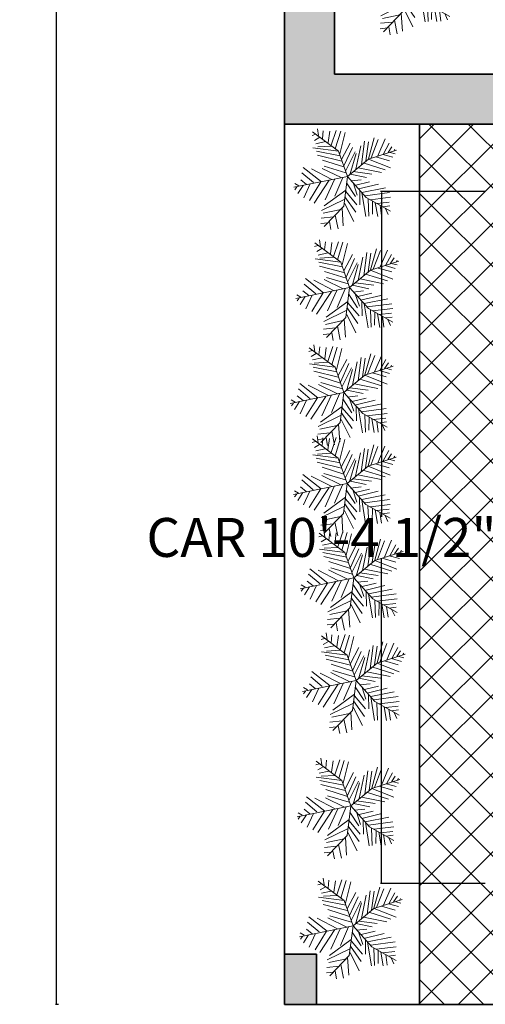
# Model space of a CAD drawing. Units: inches. Extents: x 2167 to 2589, y 1680 to 2489.
# Tile 1 of 38: x 2167 to 2251, y 1688 to 1865. Entities that reach past the tile are written whole.
import ezdxf

# ---------------------------------------------------------------- set-up
doc = ezdxf.new("R2010")
doc.units = ezdxf.units.IN
doc.header["$MEASUREMENT"] = 0
doc.layers.get('0').update_dxf_attribs({"color": 250})
for name, color, linetype, lineweight in [('A-ANNO-DIMS', 2, 'Continuous', 18), ('A-WALL-PATT', 250, 'Continuous', 13), ('C-PROP', 7, 'Continuous', 35), ('L-PLNT', 106, 'Continuous', 13), ('L-PVMT-PATT', 252, 'Continuous', 13), ('walls', 7, 'Continuous', 35)]:
    doc.layers.add(name, color=color, linetype=linetype, lineweight=lineweight)
doc.styles.get("Standard").update_dxf_attribs({"font": 'arial.ttf'})
doc.dimstyles.get("Standard").update_dxf_attribs({"dimtxt": 7, "dimasz": 0.18, "dimexe": 0.18, "dimexo": 0.0625, "dimgap": 0.09, "dimtad": 0, "dimtih": 1, "dimtoh": 1, "dimdec": 1, "dimzin": 0, "dimdsep": 46, "dimlunit": 3, "dimtxsty": 'Standard', "dimcen": 0.09, "dimadec": 0, "dimazin": 0, "dimtfac": 1, "dimtdec": 1, "dimtofl": 0, "dimtmove": 0, "dimatfit": 3, "dimfxl": 1, "dimtolj": 1, "dimtzin": 0, "dimarcsym": 0})

# ---------------------------------------------------------------- blocks, each defined once
blk = doc.blocks.new('*U8')
for p, q in [((-8.737, 47.138), (-17.069, 52.711)), ((-10.186, 53.64), (-13.084, 55.962)), ((0, 0), (-10.5, 57)), ((-9.099, 51.782), (-6.563, 55.962)), ((-7.288, 39.707), (-21.778, 46.673)), ((-7.65, 43.423), (-2.578, 49.46)), ((-5.839, 35.992), (4.667, 48.067)), ((-5.114, 27.632), (10.463, 46.673)), ((-3.665, 19.273), (-27.574, 35.527)), ((-5.114, 28.097), (-24.676, 40.636)), ((-2.941, 16.486), (8.652, 37.85)), ((16.259, 5.805), (23.142, 31.348)), ((22.055, 7.198), (27.489, 32.277)), ((27, 9), (48, 36)), ((27.127, 9.056), (31.112, 35.992)), ((35.096, 32.741), (37.27, 22.524)), ((38.719, 34.134), (41.979, 28.561)), ((44.153, 36.456), (45.239, 32.741)), ((-31.5, 4.5), (-52.5, 25.5)), ((-48.585, 21.131), (-49.309, 29.026)), ((-43.513, 28.561), (-42.427, 15.558)), ((-38.442, 26.239), (-34.819, 7.663)), ((-35.544, 28.097), (-24.314, 3.947)), ((-14.533, 2.09), (-30.834, 25.31)), ((-24.314, 23.917), (-2.941, 13.7)), ((-1.129, 6.734), (9.014, 26.704)), ((3.942, 1.625), (11.187, 24.381)), ((10.101, 3.483), (17.708, 26.239)), ((31.836, 30.883), (32.561, 16.486)), ((40.53, 25.775), (48.862, 24.846)), ((43.791, 29.954), (51.036, 30.883)), ((-47.498, 19.737), (-55.83, 18.344)), ((-40.615, 13.7), (-55.105, 10.913)), ((-20.691, 13.7), (-1.129, 4.876)), ((29.662, 12.307), (48.137, 6.269)), ((33.285, 16.486), (48.862, 10.913)), ((36.183, 19.737), (48.137, 17.88)), ((-33.37, 6.269), (-52.207, 5.34)), ((-28.299, 3.483), (-47.86, -5.805)), ((-21.416, 3.018), (-38.079, -8.128)), ((0, 0), (-31.5, 4.5)), ((-15.982, 2.09), (-30.11, -9.521)), ((0, 0), (-22.5, -19.5)), ((-6.563, 1.161), (-21.416, -8.128)), ((0, 0), (27, 9)), ((0, 0), (18, -22.5)), ((6.478, 1.625), (26.04, -8.592)), ((11.187, 3.483), (30.749, -5.805)), ((18.07, 5.805), (35.096, -3.483)), ((24.229, 7.663), (46.688, 1.625)), ((-6.563, -5.805), (-19.967, -9.985)), ((-9.461, -8.592), (-6.201, -23.453)), ((-4.752, -3.483), (-3.665, -14.629)), ((2.493, -3.019), (-1.491, -20.202)), ((1.769, -2.555), (24.229, -9.521)), ((5.029, -6.27), (2.131, -25.775)), ((7.565, -9.056), (32.198, -14.629)), ((-17.431, -15.094), (-42.789, -18.809)), ((-22.5, -19.5), (-37.5, -45)), ((-15.257, -12.772), (-30.11, -12.772)), ((-20.691, -18.345), (-17.793, -44.352)), ((-17.069, -15.094), (-12.721, -40.172)), ((-13.446, -11.378), (-8.737, -32.741)), ((9.014, -11.378), (3.58, -35.992)), ((14.085, -16.951), (6.478, -40.172)), ((12.274, -15.094), (36.907, -18.809)), ((16.259, -19.738), (36.183, -22.989)), ((-28.299, -29.026), (-42.789, -31.348)), ((-24.314, -21.596), (-42.427, -22.06)), ((-26.849, -26.24), (-40.253, -25.775)), ((-29.023, -30.884), (-27.936, -43.887)), ((-25.038, -23.918), (-22.865, -45.281)), ((18.07, -22.524), (8.289, -45.745)), ((20.244, -30.419), (15.897, -44.816)), ((18, -22.5), (27, -52.5)), ((18.433, -22.524), (40.53, -29.026)), ((19.157, -25.311), (38.719, -33.206)), ((-30.834, -34.135), (-42.427, -35.528)), ((-34.457, -39.708), (-40.978, -42.494)), ((-32.646, -36.921), (-31.921, -44.352)), ((22.78, -37.85), (19.519, -48.532)), ((21.331, -32.741), (39.081, -40.636)), ((22.78, -38.314), (34.372, -44.816)), ((24.591, -45.745), (23.142, -50.854)), ((24.591, -43.423), (30.749, -47.603)), ((26.764, -49.925), (28.213, -50.854))]:
    blk.add_line(p, q)
blk = doc.blocks.new('*D24')
at = {"layer": 'A-ANNO-DIMS', "color": 0, "lineweight": -2, "transparency": 16777216}
for p, q in [((2174.43, 2407.69), (2173.89, 2407.69)), ((2174.07, 2407.51), (2174.07, 2051.36)), ((2174.07, 1687.87), (2174.07, 2044.03)), ((2174.43, 1687.69), (2173.89, 1687.69))]:
    blk.add_line(p, q, dxfattribs=at)
at = {"layer": 'A-ANNO-DIMS', "color": 0, "transparency": 16777216}
for points in [[(2174.04, 2407.51), (2174.1, 2407.51), (2174.07, 2407.69)], [(2174.04, 1687.87), (2174.1, 1687.87), (2174.07, 1687.69)]]:
    blk.add_solid(points, dxfattribs=at)
at = {"layer": 'Defpoints', "color": 0, "transparency": 16777216}
for p in [(2174.49, 2407.69), (2174.07, 1687.69), (2174.49, 1687.69)]:
    blk.add_point(p, dxfattribs=at)
at = {"layer": 'A-ANNO-DIMS', "color": 0, "transparency": 16777216, "insert": (2174.07, 2047.69), "char_height": 7, "attachment_point": 5}
blk.add_mtext("\\A1;60'", dxfattribs=at)
blk = doc.blocks.new('*D45')
at = {"layer": 'A-ANNO-DIMS', "color": 0, "lineweight": -2, "transparency": 16777216}
for p, q in [((2251.16, 1833.95), (2232.36, 1833.95)), ((2232.54, 1833.77), (2232.54, 1775.4)), ((2232.54, 1709.6), (2232.54, 1767.98)), ((2251.16, 1709.42), (2232.36, 1709.42))]:
    blk.add_line(p, q, dxfattribs=at)
at = {"layer": 'A-ANNO-DIMS', "color": 0, "transparency": 16777216}
for points in [[(2232.51, 1833.77), (2232.57, 1833.77), (2232.54, 1833.95)], [(2232.51, 1709.6), (2232.57, 1709.6), (2232.54, 1709.42)]]:
    blk.add_solid(points, dxfattribs=at)
at = {"layer": 'Defpoints', "color": 0, "transparency": 16777216}
for p in [(2251.22, 1833.95), (2232.54, 1709.42), (2251.22, 1709.42)]:
    blk.add_point(p, dxfattribs=at)
at = {"layer": 'A-ANNO-DIMS', "color": 0, "transparency": 16777216, "insert": (2232.54, 1771.69), "char_height": 7, "attachment_point": 5}
blk.add_mtext('\\A1;CAR 10\'-4 1/2" TYP.', dxfattribs=at)

msp = doc.modelspace()

# ---------------------------------------------------------------- hatches: boundary and pattern name
at = {"layer": 'A-WALL-PATT'}
h = msp.add_hatch(color=256, dxfattribs=at)
h.dxf.hatch_style = 1
h.paths.add_polyline_path([(2274.74, 1855.04), (2224.05, 1855.04), (2224.05, 2003.12), (2215.05, 2003.12), (2215.05, 1846.04), (2274.74, 1846.04)])
h.paths.add_polyline_path([(2354.89, 1855.04), (2330.89, 1855.04), (2330.89, 1846.04), (2354.77, 1846.04), (2354.77, 1852.04, -0.01877)])
h.paths.add_polyline_path([(2422.05, 1864.69), (2426.21, 1864.69), (2426.21, 1867.92), (2426.21, 1869.19), (2422.05, 1869.19), (2422.05, 1916.24), (2417.55, 1916.24), (2417.55, 1855.04), (2394.77, 1855.04), (2394.77, 1852.04), (2394.77, 1846.04), (2417.55, 1846.04), (2417.55, 1779.19), (2427.74, 1779.19), (2427.74, 1783.94), (2427.74, 1788.19), (2422.05, 1788.19)])
h = msp.add_hatch(color=256, dxfattribs=at)
h.dxf.hatch_style = 1
h.paths.add_polyline_path([(2220.82, 1696.69), (2215.06, 1696.69), (2215.06, 1687.69), (2220.82, 1687.69)])
at = {"layer": 'L-PVMT-PATT'}
h = msp.add_hatch(dxfattribs=at)
h.set_pattern_fill('ANSI37', color=256, scale=40)
h.paths.add_polyline_path([(2417.55, 1783.69), (2417.55, 1846.04), (2239.36, 1846.04), (2239.36, 1687.69), (2369.84, 1687.69), (2369.84, 1696.69), (2375.61, 1696.69), (2416.11, 1696.69), (2417.55, 1696.69)])

# ---------------------------------------------------------------- linework, layer by layer
at = {"layer": 'C-PROP'}
for p, q in [((2215.05, 1687.69), (2215.05, 2407.69)), ((2575.05, 1687.69), (2215.05, 1687.69))]:
    msp.add_line(p, q, dxfattribs=at)
at = {"layer": 'walls'}
for p, q in [((2224.05, 1855.04), (2224.05, 2151.19)), ((2224.05, 1855.04), (2354.89, 1855.04)), ((2215.05, 1846.04), (2417.55, 1846.04)), ((2239.36, 1846.04), (2239.36, 1687.69)), ((2220.82, 1696.69), (2215.06, 1696.69)), ((2215.06, 1696.69), (2215.06, 1687.69)), ((2220.82, 1696.69), (2220.82, 1687.69))]:
    msp.add_line(p, q, dxfattribs=at)

# ---------------------------------------------------------------- block references
at = {"layer": 'L-PLNT', "xscale": 0.1698531738429223, "yscale": 0.1698531738429223, "zscale": 0.1698531738429223, "rotation": 90.98387132377816}
for p in [(2237.04, 1871.66), (2226.39, 1836.63), (2226.79, 1816.63), (2225.77, 1797.75), (2226.35, 1781.38), (2227.56, 1764.42), (2227.96, 1745.94), (2227, 1723.4), (2227.4, 1701.81)]:
    msp.add_blockref('*U8', p, dxfattribs=at)

# ---------------------------------------------------------------- dimensions: what is measured, and where the dimension line sits
at = {"layer": 'A-ANNO-DIMS'}
dim = msp.add_linear_dim(base=(2174.07, 1687.69), p1=(2174.49, 2407.69), p2=(2174.49, 1687.69), angle=90, dimstyle='Standard', override={"dimclrd": 0, "dimclre": 0, "dimclrt": 0}, dxfattribs=at)
dim.commit()
dim.dimension.update_dxf_attribs({"geometry": '*D24', "text_midpoint": (2174.07, 2047.69)})
dim = msp.add_linear_dim(base=(2232.54, 1709.42), p1=(2251.22, 1833.95), p2=(2251.22, 1709.42), angle=270, text='CAR <> TYP.', dimstyle='Standard', override={"dimdec": 1, "dimlfac": 1, "dimrnd": 0, "dimzin": 1, "dimdsep": 46, "dimlunit": 4, "dimfrac": 2}, dxfattribs=at)
dim.commit()
dim.dimension.update_dxf_attribs({"geometry": '*D45', "text_midpoint": (2232.54, 1771.69)})

doc.saveas('drawing.dxf')
